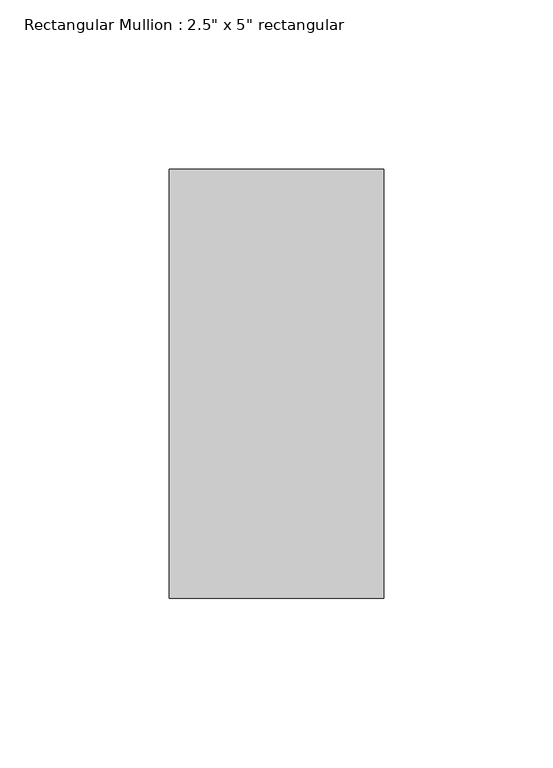
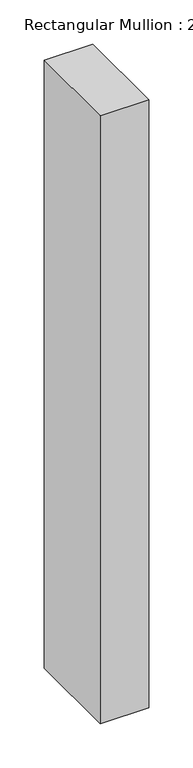
"""IFC4 building model written with IfcOpenShell, lengths in millimetres: member geometry."""

from ifc_helpers import new_model, si_unit, frame, origin, place, context, project, spatial, polyline, outline, extrude, source, transform, mapped, element, save


def member_b365ec95(model_context):
    return source(origin(), model_context, "Body", "SweptSolid", [
        extrude(outline(polyline([(0.0, 63.5), (0.0, -63.5), (-63.5, -63.5), (-63.5, 63.5), (0.0, 63.5)])), frame((0.0, 0.0, -841.0290241), z_axis=(0.0, 0.0, 1.0), x_axis=(1.0, 0.0, 0.0)), (0.0, 0.0, 1.0), 841.0290241),
    ])


if __name__ == "__main__":
    model = new_model("IFC4")
    model_context = context("Model", 3, world=origin())
    ifc_project = project(units=[si_unit("LENGTHUNIT", "METRE", prefix="MILLI")], contexts=[model_context])
    site = spatial("IfcSite", under=ifc_project)
    building = spatial("IfcBuilding", under=site)
    placement = place(None, origin())
    member_shape = member_b365ec95(model_context)
    element("IfcMember", 1, ObjectType="Rectangular Mullion : 2.5\" x 5\" rectangular", at=placement, inside=building, context=model_context, shape_type="MappedRepresentation", body=[
        mapped(member_shape, transform((0.0, 0.0, 0.0), x_axis=(1.0, 0.0, 0.0), y_axis=(0.0, 1.0, 0.0), z_axis=(0.0, 0.0, 1.0))),
    ])
    save(model, "model.ifc")

# Revit data of these elements
# Type "Rectangular Mullion : 2.5\" x 5\" rectangular"
#   built-in parameter 1007304 = 0.416667 (stored number, unit not read)
#   built-in parameter 1007301 = 0.104167 (stored number, unit not read)
#   built-in parameter 1007300 = 0.104167 (stored number, unit not read)
# Element 1 (IfcMember, "Rectangular Mullion : 2.5\" x 5\" rectangular")
#   Materials on its faces: "Aluminum"
# Materials
#   "Aluminum": class "Metal", colour RGB 247 247 247, transparency 0, Description = "Aluminum 6061", Cost = 0
